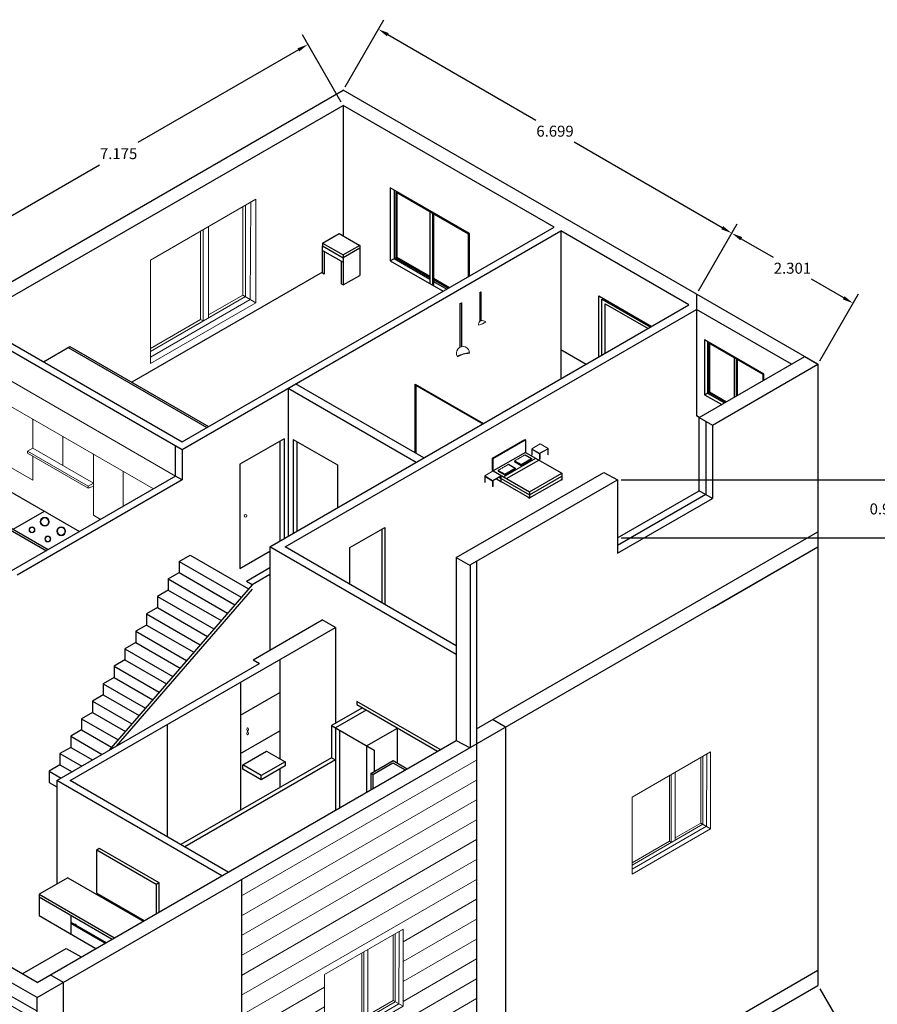
# Model space of a CAD drawing. Units: metres. Extents: x 14054 to 28215, y 4175 to 8383.
# Tile 3 of 6: x 14063.29 to 14077.36, y 4183.08 to 4199.25. Entities that reach past the tile are written whole.
import ezdxf

# ---------------------------------------------------------------- set-up
doc = ezdxf.new("R2010")
doc.units = ezdxf.units.M
for name, color, linetype, lineweight in [('A-ANNO-DIMS', 2, 'Continuous', 18), ('A-ANNO-NPLT', 9, 'Continuous', 13), ('A-ELEV-ISOM', 7, 'Continuous', 25), ('A-FURN', 8, 'Continuous', 13), ('A-GLAZ', 4, 'Continuous', 18), ('A-WALL-PATT', 8, 'Continuous', 13)]:
    doc.layers.add(name, color=color, linetype=linetype, lineweight=lineweight)
doc.styles.get("Standard").update_dxf_attribs({"font": 'arial.ttf'})
doc.dimstyles.get("Standard").update_dxf_attribs({"dimtxt": 0.18, "dimasz": 0.18, "dimexe": 0.18, "dimexo": 0.0625, "dimgap": 0.09, "dimtad": 0, "dimtih": 1, "dimtoh": 1, "dimdec": 4, "dimzin": 0, "dimdsep": 46, "dimtxsty": 'Standard', "dimcen": 0.09, "dimadec": 0, "dimazin": 0, "dimtfac": 1, "dimtdec": 4, "dimtofl": 0, "dimtmove": 0, "dimatfit": 3, "dimfxl": 1, "dimtolj": 1, "dimtzin": 0, "dimarcsym": 0})

# ---------------------------------------------------------------- blocks, each defined once
blk = doc.blocks.new('WINDOWS')
for p, q in [((14062.382, 4194.254), (14062.382, 4193.754)), ((14062.382, 4193.754), (14062.017, 4193.543)), ((14062.382, 4193.754), (14065.846, 4191.754)), ((14062.017, 4193.543), (14065.481, 4191.543)), ((14062.017, 4193.543), (14062.017, 4192.543)), ((14062.512, 4193.258), (14062.512, 4192.258)), ((14063.007, 4192.972), (14063.007, 4191.972)), ((14063.502, 4192.686), (14063.502, 4192.214)), ((14062.017, 4192.543), (14063.502, 4191.686)), ((14062.187, 4192.446), (14062.187, 4192.046)), ((14063.997, 4192.4), (14063.997, 4191.928)), ((14063.502, 4192.214), (14063.414, 4192.164)), ((14063.502, 4192.214), (14064.498, 4191.639)), ((14063.414, 4192.164), (14064.411, 4191.589)), ((14063.414, 4192.164), (14063.414, 4192.132)), ((14063.414, 4192.132), (14064.411, 4191.557)), ((14063.502, 4192.082), (14063.502, 4191.686)), ((14064.498, 4192.111), (14064.498, 4191.111)), ((14064.987, 4191.829), (14064.987, 4191.258)), ((14064.498, 4191.639), (14064.411, 4191.589)), ((14064.411, 4191.589), (14064.411, 4191.557)), ((14064.411, 4191.557), (14064.498, 4191.589)), ((14064.498, 4191.111), (14064.615, 4191.043))]:
    blk.add_line(p, q)
for p in [(14062.512, 4193.258), (14063.007, 4192.972), (14063.502, 4192.686), (14064.492, 4192.115), (14064.987, 4191.829)]:
    blk.add_point(p)
blk = doc.blocks.new('WINDOW 1')
for p, q in [((14073.717, 4186.789), (14075.449, 4187.789)), ((14075.276, 4187.689), (14075.276, 4186.189)), ((14075.365, 4187.74), (14075.356, 4186.143)), ((14075.449, 4187.789), (14075.449, 4186.089)), ((14075.233, 4187.664), (14075.233, 4186.214)), ((14074.54, 4187.264), (14074.54, 4185.814)), ((14074.583, 4187.289), (14074.583, 4185.789)), ((14074.67, 4187.34), (14074.67, 4185.84)), ((14073.717, 4185.089), (14073.717, 4186.789)), ((14075.276, 4186.189), (14073.717, 4185.289)), ((14075.356, 4186.143), (14073.717, 4185.197)), ((14075.449, 4186.089), (14073.717, 4185.089)), ((14075.233, 4186.214), (14074.67, 4185.889)), ((14075.233, 4186.214), (14075.449, 4186.089)), ((14074.54, 4185.814), (14073.717, 4185.339)), ((14074.583, 4185.789), (14074.54, 4185.814))]:
    blk.add_line(p, q)
blk = doc.blocks.new('TABLE')
for p, q in [((14070.836, 4191.718), (14070.938, 4191.777)), ((14070.938, 4191.777), (14071.033, 4191.722)), ((14070.836, 4191.718), (14070.93, 4191.663)), ((14070.836, 4191.718), (14070.836, 4191.711)), ((14070.836, 4191.711), (14070.93, 4191.656)), ((14070.836, 4191.711), (14070.836, 4191.643)), ((14070.841, 4191.64), (14070.836, 4191.643)), ((14070.841, 4191.708), (14070.841, 4191.64)), ((14071.033, 4191.722), (14070.93, 4191.663)), ((14071.033, 4191.715), (14070.93, 4191.656)), ((14070.93, 4191.656), (14070.93, 4191.663)), ((14070.93, 4191.589), (14070.93, 4191.656)), ((14070.937, 4191.66), (14070.937, 4191.592)), ((14071.027, 4191.644), (14071.027, 4191.712)), ((14071.033, 4191.648), (14071.027, 4191.644)), ((14071.033, 4191.722), (14071.033, 4191.715)), ((14071.033, 4191.715), (14071.033, 4191.648)), ((14070.937, 4191.592), (14070.93, 4191.589))]:
    blk.add_line(p, q)
blk = doc.blocks.new('*D11')
at = {"layer": 'A-ANNO-DIMS', "color": 0, "lineweight": -2, "transparency": 16777216}
for p, q in [((14076.421, 4183.337), (14077.057, 4182.235)), ((14076.812, 4182.301), (14070.874, 4178.873)), ((14064.306, 4175.081), (14070.244, 4178.509)), ((14063.604, 4175.937), (14064.24, 4174.835))]:
    blk.add_line(p, q, dxfattribs=at)
at = {"layer": 'A-ANNO-DIMS', "color": 0, "transparency": 16777216}
for points in [[(14076.797, 4182.327), (14076.827, 4182.275), (14076.967, 4182.391)], [(14064.291, 4175.107), (14064.321, 4175.055), (14064.15, 4174.991)]]:
    blk.add_solid(points, dxfattribs=at)
at = {"layer": 'Defpoints', "color": 0, "transparency": 16777216}
for p in [(14076.39, 4183.391), (14063.573, 4175.991), (14064.15, 4174.991)]:
    blk.add_point(p, dxfattribs=at)
at = {"layer": 'A-ANNO-DIMS', "color": 0, "transparency": 16777216, "insert": (14070.559, 4178.691), "char_height": 0.18, "attachment_point": 5}
blk.add_mtext('\\A1;14.8', dxfattribs=at)
blk = doc.blocks.new('*D72')
at = {"layer": 'A-ANNO-DIMS', "color": 0, "lineweight": -2, "transparency": 16777216}
for p, q in [((14068.564, 4197.895), (14067.928, 4198.997)), ((14067.862, 4198.752), (14065.226, 4197.23)), ((14061.96, 4195.344), (14064.596, 4196.866)), ((14062.351, 4194.308), (14061.714, 4195.41))]:
    blk.add_line(p, q, dxfattribs=at)
at = {"layer": 'A-ANNO-DIMS', "color": 0, "transparency": 16777216}
for points in [[(14067.847, 4198.777), (14067.877, 4198.726), (14068.018, 4198.842)], [(14061.945, 4195.37), (14061.975, 4195.318), (14061.804, 4195.254)]]:
    blk.add_solid(points, dxfattribs=at)
at = {"layer": 'Defpoints', "color": 0, "transparency": 16777216}
for p in [(14068.018, 4198.842), (14068.596, 4197.841), (14062.382, 4194.254)]:
    blk.add_point(p, dxfattribs=at)
at = {"layer": 'A-ANNO-DIMS', "color": 0, "transparency": 16777216, "insert": (14064.911, 4197.048), "char_height": 0.18, "attachment_point": 5}
blk.add_mtext('\\A1;7.175', dxfattribs=at)
blk = doc.blocks.new('*D73')
at = {"layer": 'A-ANNO-DIMS', "color": 0, "lineweight": -2, "transparency": 16777216}
for p, q in [((14068.627, 4198.145), (14069.263, 4199.247)), ((14069.329, 4199.002), (14071.759, 4197.599)), ((14074.819, 4195.832), (14072.389, 4197.235)), ((14074.429, 4194.796), (14075.065, 4195.898))]:
    blk.add_line(p, q, dxfattribs=at)
at = {"layer": 'A-ANNO-DIMS', "color": 0, "transparency": 16777216}
for points in [[(14069.344, 4199.027), (14069.314, 4198.976), (14069.173, 4199.092)], [(14074.834, 4195.858), (14074.804, 4195.806), (14074.975, 4195.742)]]:
    blk.add_solid(points, dxfattribs=at)
at = {"layer": 'Defpoints', "color": 0, "transparency": 16777216}
for p in [(14068.596, 4198.091), (14074.975, 4195.742), (14074.397, 4194.742)]:
    blk.add_point(p, dxfattribs=at)
at = {"layer": 'A-ANNO-DIMS', "color": 0, "transparency": 16777216, "insert": (14072.074, 4197.417), "char_height": 0.18, "attachment_point": 5}
blk.add_mtext('\\A1;6.699', dxfattribs=at)
blk = doc.blocks.new('*D74')
at = {"layer": 'A-ANNO-DIMS', "color": 0, "lineweight": -2, "transparency": 16777216}
for p, q in [((14074.429, 4194.796), (14075.065, 4195.898)), ((14075.131, 4195.652), (14075.656, 4195.349)), ((14076.812, 4194.682), (14076.286, 4194.985)), ((14076.421, 4193.645), (14077.057, 4194.747))]:
    blk.add_line(p, q, dxfattribs=at)
at = {"layer": 'A-ANNO-DIMS', "color": 0, "transparency": 16777216}
for points in [[(14075.146, 4195.678), (14075.116, 4195.626), (14074.975, 4195.742)], [(14076.827, 4194.707), (14076.797, 4194.656), (14076.967, 4194.592)]]:
    blk.add_solid(points, dxfattribs=at)
at = {"layer": 'Defpoints', "color": 0, "transparency": 16777216}
for p in [(14074.397, 4194.742), (14076.967, 4194.592), (14076.39, 4193.591)]:
    blk.add_point(p, dxfattribs=at)
at = {"layer": 'A-ANNO-DIMS', "color": 0, "transparency": 16777216, "insert": (14075.971, 4195.167), "char_height": 0.18, "attachment_point": 5}
blk.add_mtext('\\A1;2.301', dxfattribs=at)
blk = doc.blocks.new('*D75')
at = {"layer": 'A-ANNO-DIMS', "color": 0, "lineweight": -2, "transparency": 16777216}
for p, q in [((14073.161, 4191.691), (14077.725, 4191.691)), ((14077.545, 4191.511), (14077.545, 4191.397)), ((14077.545, 4190.918), (14077.545, 4191.033)), ((14073.161, 4190.738), (14077.725, 4190.738))]:
    blk.add_line(p, q, dxfattribs=at)
at = {"layer": 'A-ANNO-DIMS', "color": 0, "transparency": 16777216}
for points in [[(14077.515, 4191.511), (14077.575, 4191.511), (14077.545, 4191.691)], [(14077.515, 4190.918), (14077.575, 4190.918), (14077.545, 4190.738)]]:
    blk.add_solid(points, dxfattribs=at)
at = {"layer": 'Defpoints', "color": 0, "transparency": 16777216}
for p in [(14073.099, 4191.691), (14073.099, 4190.738), (14077.545, 4190.738)]:
    blk.add_point(p, dxfattribs=at)
at = {"layer": 'A-ANNO-DIMS', "color": 0, "transparency": 16777216, "insert": (14077.545, 4191.215), "char_height": 0.18, "attachment_point": 5}
blk.add_mtext('\\A1;0.953', dxfattribs=at)

msp = doc.modelspace()

# ---------------------------------------------------------------- hatches: boundary and pattern name
at = {"layer": 'A-WALL-PATT'}
h = msp.add_hatch(dxfattribs=at)
h.set_pattern_fill('ANSI38', color=256, scale=0.092, angle=105)
h.paths.add_polyline_path([(14055.7785, 4187.4672), (14055.7785, 4180.7413), (14058.8262, 4178.9816), (14058.8262, 4185.7075)])
h.paths.add_polyline_path([(14058.0676, 4184.5273), (14058.0676, 4183.2595), (14056.6953, 4184.0519), (14056.6953, 4185.3196)], flags=16)
h.paths.add_polyline_path([(14056.7604, 4184.0895), (14056.7893, 4184.1061), (14056.7893, 4185.2436), (14058.0488, 4184.5164), (14058.0488, 4183.401), (14057.4455, 4183.7494), (14057.4455, 4183.6399), (14057.4272, 4183.6293), (14057.4272, 4184.8753), (14057.3815, 4184.9017), (14057.3815, 4183.7309)], flags=0)
h.paths.add_polyline_path([(14063.5727, 4180.0812), (14062.8942, 4180.4729), (14061.5218, 4181.2653), (14060.8587, 4181.6535), (14060.8401, 4177.8243), (14063.5727, 4176.2413)])
h.paths.add_polyline_path([(14060.8494, 4184.7636), (14060.9576, 4184.8261), (14058.9345, 4185.9941), (14058.9345, 4178.9191), (14060.8494, 4177.8136)])
h.paths.add_polyline_path([(14060.7529, 4181.7978), (14060.7529, 4181.7242), (14060.7529, 4178.127), (14059.0613, 4179.1036), (14059.0613, 4182.7744)], flags=16)
h.paths.add_polyline_path([(14059.2399, 4179.1538), (14059.2399, 4182.5977), (14060.0427, 4182.1342), (14060.0427, 4178.6903)], flags=0)
h.paths.add_polyline_path([(14060.215, 4182.0347), (14060.7096, 4181.7492), (14060.7096, 4178.3053), (14060.215, 4178.5908)], flags=0)
edge = h.paths.add_edge_path(flags=0)
edge.add_ellipse((14059.9307, 4180.1763), major_axis=(-0.0333, 0.0192), ratio=0.8810932, start_angle=0, end_angle=360)
h = msp.add_hatch(dxfattribs=at)
h.set_pattern_fill('ANSI31', color=256, scale=0.089, angle=165)
h.paths.add_polyline_path([(14070.7875, 4187.3567), (14066.9286, 4185.1288), (14066.9286, 4178.1788), (14070.7875, 4180.4067)])
h.paths.add_polyline_path([(14069.5808, 4184.3152), (14069.5808, 4183.05), (14068.2917, 4182.3057), (14068.2917, 4183.5709)], flags=16)
h.paths.add_polyline_path([(14069.4519, 4183.1244), (14069.0007, 4182.8639), (14069.0007, 4182.9011), (14069.4197, 4183.143)], flags=0)
h = msp.add_hatch(dxfattribs=at)
h.set_pattern_fill('ANSI31', color=256, scale=0.089, angle=105)
h.paths.add_polyline_path([(14063.5727, 4182.9672), (14060.8494, 4184.5395), (14060.8494, 4181.6535), (14061.5218, 4181.2653), (14061.5218, 4182.533), (14062.8942, 4181.7407), (14062.8942, 4180.4729), (14063.5727, 4180.0812)])

# ---------------------------------------------------------------- linework, layer by layer
at = {"layer": 'A-ANNO-NPLT'}
msp.add_point((14063.9968, 4192.4004), dxfattribs=at)
at = {"layer": 'A-ELEV-ISOM'}
for p, q in [((14055.995, 4190.8163), (14068.5957, 4198.0913)), ((14076.3899, 4193.5913), (14068.5957, 4198.0913)), ((14062.4902, 4194.3163), (14068.5957, 4197.8413)), ((14072.0598, 4195.8413), (14068.5957, 4197.8413)), ((14068.5957, 4197.8413), (14068.5957, 4195.6998)), ((14070.6694, 4195.7385), (14069.3703, 4196.4885)), ((14069.3703, 4196.4885), (14069.3703, 4195.2885)), ((14069.4319, 4196.4529), (14069.4319, 4195.3241)), ((14069.4593, 4196.4166), (14069.4593, 4195.3399)), ((14070.6515, 4195.7282), (14069.4593, 4196.4166)), ((14069.4774, 4196.4061), (14069.4774, 4195.3503)), ((14070.0198, 4196.0929), (14070.0198, 4194.9135)), ((14070.0631, 4196.0679), (14070.0631, 4194.8885)), ((14070.0805, 4196.0579), (14070.0805, 4194.8985)), ((14065.9543, 4192.3163), (14072.0598, 4195.8413)), ((14065.9543, 4192.1913), (14072.168, 4195.7788)), ((14074.2724, 4194.5638), (14072.168, 4195.7788)), ((14072.168, 4195.7788), (14072.168, 4193.3489)), ((14068.2589, 4195.5789), (14068.5321, 4195.7366)), ((14068.5321, 4195.7366), (14068.8682, 4195.5425)), ((14070.6515, 4195.0282), (14070.6515, 4195.7282)), ((14070.6694, 4195.0385), (14070.6694, 4195.7385)), ((14068.2589, 4195.5789), (14068.595, 4195.3848)), ((14068.2589, 4195.5789), (14068.2589, 4195.5335)), ((14068.2589, 4195.5335), (14068.595, 4195.3395)), ((14068.2589, 4195.0861), (14068.2589, 4195.5335)), ((14068.2589, 4195.46), (14068.595, 4195.266)), ((14068.2836, 4195.4458), (14068.2836, 4195.0719)), ((14068.8682, 4195.5425), (14068.595, 4195.3848)), ((14068.8682, 4195.4972), (14068.595, 4195.3395)), ((14068.8682, 4195.5425), (14068.8682, 4195.4972)), ((14068.8682, 4195.4972), (14068.8682, 4195.0498)), ((14068.5703, 4194.9063), (14068.5703, 4195.2802)), ((14068.595, 4195.3848), (14068.595, 4195.3395)), ((14068.595, 4195.3395), (14068.595, 4194.8921)), ((14069.3703, 4195.2885), (14069.4774, 4195.3503)), ((14069.3703, 4195.2885), (14070.2363, 4194.7885)), ((14069.4319, 4195.3241), (14070.0198, 4194.9847)), ((14069.4593, 4195.3399), (14070.0198, 4195.0163)), ((14069.4774, 4195.3503), (14070.0198, 4195.0372)), ((14068.2589, 4195.1038), (14065.1255, 4193.2947)), ((14068.2836, 4195.0719), (14068.2589, 4195.0861)), ((14068.595, 4194.8921), (14068.8682, 4195.0498)), ((14070.0805, 4195.0022), (14070.3434, 4194.8503)), ((14070.0805, 4194.9813), (14070.3253, 4194.8399)), ((14070.0805, 4194.9497), (14070.298, 4194.8241)), ((14068.595, 4194.8921), (14068.5703, 4194.9063)), ((14070.0631, 4194.8885), (14070.0805, 4194.8985)), ((14070.8402, 4194.7666), (14070.861, 4194.7786)), ((14070.8402, 4194.7666), (14070.8402, 4194.2979)), ((14070.861, 4194.3098), (14070.861, 4194.7786)), ((14072.7947, 4193.7107), (14072.7947, 4194.7144)), ((14072.7947, 4194.7144), (14073.6639, 4194.2125)), ((14072.8405, 4193.7371), (14072.8405, 4194.6593)), ((14072.8405, 4194.6593), (14073.6391, 4194.1982)), ((14074.3974, 4194.7416), (14074.3974, 4192.7428)), ((14067.3937, 4190.5924), (14074.2724, 4194.5638)), ((14067.6437, 4190.5924), (14074.3974, 4194.4916)), ((14070.5109, 4194.583), (14070.5109, 4193.8679)), ((14070.5389, 4194.5992), (14070.5389, 4193.8786)), ((14072.8959, 4193.7691), (14072.8959, 4194.5826)), ((14072.8959, 4194.5826), (14073.6004, 4194.1759)), ((14075.9569, 4193.5913), (14074.3974, 4194.4916)), ((14062.4902, 4194.3163), (14065.9543, 4192.3163)), ((14070.8402, 4194.2979), (14070.861, 4194.3098)), ((14062.3819, 4194.2538), (14065.9543, 4192.1913)), ((14075.5034, 4193.4278), (14074.5303, 4193.9896)), ((14074.5303, 4193.9896), (14074.5303, 4193.0907)), ((14063.6782, 4193.6303), (14064.1113, 4193.8803)), ((14064.0839, 4193.8645), (14066.3599, 4192.5505)), ((14064.1113, 4193.8803), (14066.3873, 4192.5663)), ((14072.168, 4193.8328), (14072.5871, 4193.5909)), ((14074.5764, 4193.963), (14074.5764, 4193.1174)), ((14074.5969, 4193.9357), (14074.5969, 4193.1292)), ((14075.4901, 4193.4201), (14074.5969, 4193.9357)), ((14074.6105, 4193.9279), (14074.6105, 4193.137)), ((14074.4413, 4192.7163), (14076.1734, 4193.7163)), ((14075.0168, 4193.6933), (14075.0168, 4193.0485)), ((14075.0493, 4193.6746), (14075.0493, 4193.0673)), ((14075.0622, 4193.6671), (14075.0622, 4193.0747)), ((14076.1734, 4193.7163), (14076.3899, 4193.5913)), ((14074.6578, 4192.5913), (14076.3899, 4193.5913)), ((14076.3899, 4193.5913), (14076.3899, 4190.5913)), ((14075.4901, 4193.3217), (14075.4901, 4193.4201)), ((14075.5034, 4193.3294), (14075.5034, 4193.4278)), ((14069.7963, 4191.9795), (14067.6919, 4193.1945)), ((14067.6919, 4193.1945), (14067.6919, 4190.7646)), ((14069.9213, 4192.0517), (14067.8169, 4193.2666)), ((14069.7798, 4192.1334), (14069.7798, 4193.2657)), ((14069.7798, 4193.2657), (14070.9018, 4192.6179)), ((14069.7933, 4193.2434), (14070.8893, 4192.6106)), ((14069.7933, 4192.1256), (14069.7933, 4193.2434)), ((14074.5303, 4193.0907), (14074.6105, 4193.137)), ((14074.5303, 4193.0907), (14074.8101, 4192.9292)), ((14074.5764, 4193.1174), (14074.8562, 4192.9558)), ((14074.5969, 4193.1292), (14074.8767, 4192.9676)), ((14074.6105, 4193.137), (14074.8903, 4192.9755)), ((14074.4413, 4192.7163), (14074.3974, 4192.7428)), ((14074.4413, 4191.5132), (14074.4413, 4192.7163)), ((14074.4413, 4192.7163), (14074.6578, 4192.5913)), ((14074.5496, 4192.6538), (14074.5496, 4191.4507)), ((14074.6578, 4192.5913), (14074.6578, 4191.3882)), ((14067.6262, 4192.3666), (14066.903, 4191.949)), ((14067.6262, 4192.3666), (14067.6262, 4190.7267)), ((14065.846, 4191.7538), (14065.846, 4192.2538)), ((14067.5562, 4192.3261), (14067.5562, 4190.6862)), ((14067.7759, 4192.356), (14068.5011, 4191.9373)), ((14067.7759, 4192.356), (14067.7759, 4190.8131)), ((14067.838, 4192.3202), (14067.838, 4190.8489)), ((14071.0498, 4192.0485), (14071.5783, 4192.3536)), ((14071.0605, 4192.0423), (14071.589, 4192.3474)), ((14071.5783, 4192.3536), (14071.589, 4192.3474)), ((14071.589, 4192.3474), (14071.589, 4192.144)), ((14062.1865, 4192.0456), (14064.269, 4190.8433)), ((14065.9543, 4192.1913), (14065.9543, 4191.6913)), ((14071.0498, 4191.8451), (14071.0498, 4192.0485)), ((14071.0605, 4192.0423), (14071.0498, 4192.0485)), ((14071.589, 4192.144), (14071.0605, 4191.8389)), ((14071.0605, 4191.8389), (14071.0605, 4192.0423)), ((14071.2285, 4191.7419), (14071.757, 4192.047)), ((14071.5184, 4191.9427), (14071.6903, 4192.0419)), ((14071.583, 4192.1038), (14071.6903, 4192.0419)), ((14071.589, 4192.144), (14072.1834, 4191.8008)), ((14071.6903, 4192.0419), (14071.6903, 4192.0295)), ((14066.903, 4191.949), (14066.903, 4190.2376)), ((14068.5011, 4191.9373), (14068.5011, 4191.2318)), ((14071.248, 4191.7866), (14071.4199, 4191.8858)), ((14071.2788, 4191.7129), (14071.8072, 4192.018)), ((14071.3126, 4191.9477), (14071.4199, 4191.8858)), ((14071.4111, 4192.0046), (14071.5184, 4191.9427)), ((14071.4111, 4192.0046), (14071.4111, 4191.9922)), ((14071.4111, 4191.9922), (14071.5184, 4191.9302)), ((14071.4199, 4191.8858), (14071.4199, 4191.8734)), ((14071.5184, 4191.9302), (14071.6903, 4192.0295)), ((14071.5184, 4191.9302), (14071.5184, 4191.9427)), ((14065.846, 4191.7538), (14063.1397, 4190.1913)), ((14065.9543, 4191.6913), (14065.846, 4191.7538)), ((14070.4541, 4190.4158), (14072.8739, 4191.8121)), ((14071.0498, 4191.8451), (14071.0605, 4191.8389)), ((14071.0605, 4191.8389), (14071.6549, 4191.4957)), ((14071.1408, 4191.8485), (14071.248, 4191.7866)), ((14071.1408, 4191.8485), (14071.1408, 4191.8361)), ((14071.1408, 4191.8361), (14071.248, 4191.7741)), ((14071.1551, 4191.7342), (14071.1817, 4191.7189)), ((14071.248, 4191.7741), (14071.4199, 4191.8734)), ((14071.248, 4191.7741), (14071.248, 4191.7866)), ((14071.6549, 4191.4957), (14072.1834, 4191.8008)), ((14071.6549, 4191.4457), (14072.1834, 4191.7508)), ((14072.1834, 4191.8008), (14072.1834, 4191.7008)), ((14072.8739, 4191.8121), (14073.099, 4191.6913)), ((14065.9543, 4191.6913), (14063.248, 4190.1288)), ((14070.6792, 4190.295), (14073.099, 4191.6913)), ((14071.1118, 4191.7092), (14071.1817, 4191.6689)), ((14071.1901, 4191.7141), (14071.6549, 4191.4457)), ((14071.1901, 4191.6641), (14071.6549, 4191.3957)), ((14071.6549, 4191.3957), (14072.1834, 4191.7008)), ((14072.1834, 4191.6894), (14072.1735, 4191.6951)), ((14072.1834, 4191.7008), (14072.1834, 4191.6894)), ((14073.099, 4191.6913), (14073.099, 4190.4882)), ((14062.1761, 4191.4597), (14063.7564, 4190.5473)), ((14062.1761, 4191.4245), (14063.7259, 4190.5297)), ((14071.6369, 4191.3978), (14071.6369, 4191.4061)), ((14071.6549, 4191.3874), (14071.6369, 4191.3978)), ((14071.6549, 4191.4957), (14071.6549, 4191.3957)), ((14071.6549, 4191.3957), (14071.6549, 4191.3874)), ((14073.099, 4190.7382), (14074.4413, 4191.5132)), ((14074.5496, 4191.4507), (14073.099, 4190.6132)), ((14074.6578, 4191.3882), (14074.4413, 4191.5132)), ((14073.099, 4190.4882), (14074.6578, 4191.3882)), ((14063.1795, 4190.8803), (14063.6922, 4191.1763)), ((14068.7054, 4190.5795), (14069.2802, 4190.9114)), ((14069.2802, 4190.9114), (14069.2802, 4189.6476)), ((14069.2309, 4190.8829), (14069.2309, 4189.6761)), ((14070.7875, 4187.6067), (14076.3899, 4190.8413)), ((14063.5727, 4183.1913), (14076.3899, 4190.5913)), ((14070.4541, 4188.8255), (14067.3937, 4190.5924)), ((14067.3937, 4190.5924), (14067.3937, 4188.8987)), ((14070.4541, 4188.9698), (14067.6437, 4190.5924)), ((14071.2638, 4190.6325), (14071.2638, 4190.6323)), ((14074.6578, 4189.5913), (14076.3899, 4190.5913)), ((14076.3899, 4190.5913), (14076.3899, 4183.3913)), ((14065.9049, 4190.3536), (14066.0829, 4190.4564)), ((14066.0829, 4190.4564), (14067.0425, 4189.9024)), ((14066.903, 4190.2376), (14067.3937, 4190.5209)), ((14068.7054, 4189.9795), (14068.7054, 4190.5795)), ((14065.9049, 4190.3536), (14066.924, 4189.7652)), ((14065.9049, 4190.3536), (14065.9049, 4190.1695)), ((14070.4541, 4190.4158), (14070.4541, 4187.415)), ((14070.4541, 4190.4158), (14070.6792, 4190.2859)), ((14070.6792, 4190.295), (14070.6792, 4187.2942)), ((14070.7875, 4190.3575), (14070.7875, 4180.4067)), ((14065.7269, 4190.0667), (14065.9049, 4190.1695)), ((14065.9049, 4190.1695), (14066.8179, 4189.6423)), ((14065.9049, 4190.1695), (14066.7713, 4189.6692)), ((14067.3937, 4190.2457), (14067.0101, 4190.0242)), ((14067.3937, 4190.1397), (14067.1019, 4189.9712)), ((14067.1019, 4189.9712), (14064.7492, 4187.2466)), ((14065.7269, 4190.0667), (14066.6995, 4189.5052)), ((14065.7269, 4190.0667), (14065.7269, 4189.8825)), ((14067.1019, 4189.9712), (14067.0101, 4190.0242)), ((14067.1019, 4189.8997), (14064.8724, 4187.3177)), ((14065.7269, 4189.8825), (14065.5489, 4189.7798)), ((14065.5489, 4189.7798), (14066.4749, 4189.2451)), ((14065.5489, 4189.7798), (14065.5489, 4189.5956)), ((14065.7269, 4189.8825), (14066.5933, 4189.3823)), ((14065.7269, 4189.8825), (14066.5933, 4189.3823)), ((14065.5489, 4189.5956), (14065.3709, 4189.4928)), ((14065.3709, 4189.4928), (14066.2504, 4188.9851)), ((14065.3709, 4189.4928), (14065.3709, 4189.3086)), ((14065.5489, 4189.5956), (14066.3688, 4189.1222)), ((14065.3709, 4189.3086), (14065.1929, 4189.2059)), ((14065.3709, 4189.3086), (14066.1442, 4188.8622)), ((14067.1171, 4188.739), (14068.2516, 4189.394)), ((14068.4686, 4189.2687), (14068.2516, 4189.394)), ((14064.1133, 4186.7541), (14068.4686, 4189.2687)), ((14065.1929, 4189.2059), (14066.0258, 4188.725)), ((14065.1929, 4189.2059), (14065.1929, 4189.0217)), ((14068.4686, 4189.2687), (14068.4686, 4187.6936)), ((14065.1929, 4189.0217), (14065.0149, 4188.9189)), ((14065.1929, 4189.0217), (14065.9197, 4188.6021)), ((14065.0149, 4188.9189), (14065.8012, 4188.4649)), ((14065.0149, 4188.9189), (14065.0149, 4188.7348)), ((14063.8965, 4186.7543), (14067.2256, 4188.6763)), ((14065.0149, 4188.7348), (14064.8369, 4188.632)), ((14065.0149, 4188.7348), (14065.6951, 4188.342)), ((14067.1171, 4188.739), (14067.2256, 4188.6763)), ((14067.5552, 4188.7413), (14067.5552, 4187.1123)), ((14064.8369, 4188.632), (14065.5767, 4188.2049)), ((14064.8369, 4188.632), (14064.8369, 4188.4478)), ((14064.8369, 4188.4478), (14064.6589, 4188.3451)), ((14064.6589, 4188.3451), (14065.3521, 4187.9448)), ((14064.6589, 4188.3451), (14064.6589, 4188.1609)), ((14064.8369, 4188.4478), (14065.4705, 4188.082)), ((14066.9135, 4188.3708), (14066.9135, 4186.2691)), ((14064.6589, 4188.1609), (14064.4809, 4188.0581)), ((14064.6589, 4188.1609), (14065.246, 4187.8219)), ((14066.9135, 4187.8312), (14067.5552, 4188.2017)), ((14064.4809, 4188.0581), (14065.1276, 4187.6848)), ((14064.4809, 4188.0581), (14064.4809, 4187.8739)), ((14070.1907, 4187.2629), (14068.8222, 4188.053)), ((14068.8222, 4188.053), (14068.8222, 4188.0015)), ((14068.8222, 4188.0015), (14070.146, 4187.2371)), ((14064.4809, 4187.8739), (14064.3029, 4187.7712)), ((14064.4809, 4187.8739), (14065.0214, 4187.5619)), ((14068.912, 4187.9496), (14068.4052, 4187.657)), ((14068.9754, 4187.913), (14068.4686, 4187.6204)), ((14064.3029, 4187.7712), (14064.903, 4187.4247)), ((14064.3029, 4187.7712), (14064.3029, 4187.587)), ((14065.7061, 4187.6737), (14065.7061, 4185.8346)), ((14071.2638, 4187.6317), (14071.0473, 4187.7567)), ((14064.3029, 4187.587), (14064.1249, 4187.4842)), ((14064.3029, 4187.587), (14064.7969, 4187.3018)), ((14066.9135, 4187.2024), (14067.5552, 4187.5728)), ((14068.4052, 4187.657), (14069.1041, 4187.2535)), ((14068.4052, 4187.657), (14068.4052, 4187.1304)), ((14068.4686, 4187.6204), (14068.4686, 4186.2687)), ((14068.5346, 4187.5823), (14068.5346, 4186.3068)), ((14068.9806, 4187.3248), (14069.4874, 4187.6174)), ((14069.4841, 4187.6193), (14069.4841, 4187.0451)), ((14071.2638, 4187.6317), (14071.2638, 4180.6817)), ((14063.572, 4183.4416), (14070.4541, 4187.415)), ((14064.1249, 4187.4842), (14064.6429, 4187.1852)), ((14064.1249, 4187.4842), (14064.1249, 4187.3001)), ((14070.4541, 4187.415), (14070.6792, 4187.2942)), ((14064.1249, 4187.3001), (14063.9469, 4187.1973)), ((14063.9469, 4187.1973), (14064.3054, 4186.9903)), ((14063.9469, 4187.1973), (14063.9469, 4187.0131)), ((14064.1249, 4187.3001), (14064.4834, 4187.0931)), ((14064.1249, 4187.3001), (14064.4834, 4187.0931)), ((14066.95, 4187.0109), (14067.3404, 4187.2363)), ((14067.3404, 4187.2363), (14067.6428, 4187.0617)), ((14068.9806, 4187.3248), (14068.9806, 4186.5643)), ((14069.1041, 4187.2535), (14069.1041, 4186.9023)), ((14068.4052, 4187.1304), (14065.9334, 4185.7033)), ((14068.4686, 4187.0938), (14065.9968, 4185.6667)), ((14067.6428, 4187.0617), (14067.2525, 4186.8363)), ((14067.6428, 4187.0617), (14067.6428, 4186.9949)), ((14068.4052, 4187.1304), (14068.4686, 4187.0938)), ((14069.0516, 4186.872), (14069.4178, 4187.0834)), ((14069.0821, 4186.8544), (14069.4133, 4187.0457)), ((14069.4133, 4187.0457), (14069.6139, 4186.9299)), ((14069.4178, 4187.0834), (14069.6488, 4186.95)), ((14063.9469, 4187.0131), (14063.7689, 4186.9103)), ((14063.7689, 4186.9103), (14063.9679, 4186.7955)), ((14063.7689, 4186.9103), (14063.7689, 4186.7262)), ((14063.9469, 4187.0131), (14064.1459, 4186.8982)), ((14067.2525, 4186.8363), (14066.95, 4187.0109)), ((14066.95, 4186.9441), (14066.95, 4187.0109)), ((14067.2525, 4186.7695), (14066.95, 4186.9441)), ((14067.6428, 4186.9949), (14067.2525, 4186.7695)), ((14067.5552, 4186.9443), (14067.5552, 4186.6396)), ((14069.0821, 4186.8544), (14069.0516, 4186.872)), ((14069.0516, 4186.872), (14069.0516, 4186.6053)), ((14063.572, 4183.4416), (14057.727, 4186.8163)), ((14063.7689, 4186.7262), (14063.8965, 4186.6525)), ((14063.7689, 4186.7262), (14063.8965, 4186.6525)), ((14066.6031, 4185.1916), (14063.8965, 4186.7543)), ((14063.8965, 4186.7543), (14063.8965, 4185.0573)), ((14066.7114, 4185.2541), (14064.1133, 4186.7541)), ((14067.2525, 4186.7695), (14067.2525, 4186.8363)), ((14069.0821, 4186.8544), (14069.0821, 4186.6229)), ((14064.5508, 4185.6196), (14064.5941, 4185.6446)), ((14064.5508, 4184.9089), (14064.5508, 4185.6196)), ((14064.5508, 4185.6196), (14065.5298, 4185.0544)), ((14064.5941, 4185.6446), (14065.5731, 4185.0794)), ((14064.0755, 4185.1606), (14063.6046, 4184.8888)), ((14064.0755, 4185.1606), (14065.3125, 4184.4465)), ((14066.9286, 4185.1288), (14066.9286, 4178.1788)), ((14065.5298, 4185.0544), (14065.5731, 4185.0794)), ((14065.5298, 4185.0544), (14065.5298, 4184.572)), ((14065.5731, 4185.0794), (14065.5731, 4184.597)), ((14063.5727, 4183.1913), (14060.8494, 4184.7636)), ((14063.6046, 4184.8888), (14064.8416, 4184.1746)), ((14063.6046, 4184.8888), (14063.6046, 4184.5399)), ((14063.6046, 4184.8468), (14064.8052, 4184.1536)), ((14064.5508, 4184.9089), (14065.3321, 4184.4578)), ((14063.5727, 4182.9672), (14060.8494, 4184.5395)), ((14063.6046, 4184.5399), (14064.5394, 4184.0002)), ((14064.1253, 4184.5461), (14064.1253, 4184.2393)), ((14064.1253, 4184.4296), (14064.7043, 4184.0954)), ((14064.1253, 4184.4154), (14064.6854, 4184.0921)), ((14064.1902, 4184.3922), (14064.1902, 4184.4056)), ((14064.1902, 4184.4056), (14064.2096, 4184.3945)), ((14064.2096, 4184.3945), (14064.2096, 4184.381)), ((14063.3269, 4183.5832), (14064.0498, 4184.0006)), ((14064.0498, 4184.0006), (14064.295, 4183.859)), ((14063.5727, 4176.2413), (14076.3899, 4183.6413)), ((14064.0057, 4183.4413), (14063.7885, 4183.5666)), ((14063.5727, 4175.9913), (14076.3899, 4183.3913)), ((14064.0057, 4176.2413), (14064.0057, 4183.4413)), ((14063.5727, 4175.9913), (14063.5727, 4183.1913))]:
    msp.add_line(p, q, dxfattribs=at)
at = {"layer": 'A-FURN'}
for centre, radius in [((14063.6993, 4191.0041), 0.0735), ((14066.9925, 4191.1028), 0.0218), ((14063.4894, 4190.8707), 0.0478), ((14063.4894, 4190.8707), 0.0407), ((14063.6993, 4191.0041), 0.0624), ((14063.9684, 4190.8487), 0.0735), ((14063.9684, 4190.8487), 0.0624), ((14063.748, 4190.7214), 0.0478), ((14063.748, 4190.7214), 0.0407)]:
    msp.add_circle(centre, radius, dxfattribs=at)
for centre, radius, start, end in [((14070.8385, 4194.082), 0.2289, 64.41331, 84.37459), ((14070.8896, 4194.2486), 0.0698, 135.11893, 192.82146), ((14070.7003, 4194.6356), 0.4204, 286.76902, 304.32774), ((14070.5633, 4193.7725), 0.1089, 359.46966, 214.04112), ((14070.6912, 4193.3441), 0.435, 92.53558, 120.5819), ((14070.6944, 4193.3371), 0.435, 92.92889, 120.5819)]:
    msp.add_arc(centre, radius, start, end, dxfattribs=at)
for centre, major_axis, ratio in [((14070.5249, 4194.5911), (-0.014, -0.0081), 0.1415216), ((14067.0289, 4187.5944), (0, 0.0266), 0.5527886), ((14067.0289, 4187.5307), (0, 0.0266), 0.5527886)]:
    msp.add_ellipse(centre, major_axis=major_axis, ratio=ratio, dxfattribs=at)
for points in [[(14071.4111, 4192.0046), (14071.4283, 4192.0145), (14071.4541, 4192.0294), (14071.4898, 4192.05), (14071.5136, 4192.0638), (14071.5373, 4192.0775), (14071.5539, 4192.087), (14071.5703, 4192.0965), (14071.578, 4192.101), (14071.583, 4192.1038)], [(14071.1408, 4191.8485), (14071.1579, 4191.8584), (14071.1837, 4191.8733), (14071.2194, 4191.8939), (14071.2432, 4191.9077), (14071.267, 4191.9214), (14071.2835, 4191.9309), (14071.2999, 4191.9404), (14071.3077, 4191.9449), (14071.3126, 4191.9477)]]:
    msp.add_open_spline(points, degree=3, knots=[0, 0, 0, 0, 0.05934304, 0.08933663, 0.12379449, 0.14166437, 0.17165796, 0.18123065, 0.19845639, 0.19845639, 0.19845639, 0.19845639], dxfattribs=at)

# ---------------------------------------------------------------- block references
at = {"layer": 'A-FURN', "xscale": 1.371911927489495, "yscale": 1.371911927489495, "zscale": 1.371911927489495}
for p in [(-5232.2556, -1558.4642), (-5233.0276, -1558.9099)]:
    msp.add_blockref('TABLE', p, dxfattribs=at)
at = {"layer": 'A-GLAZ'}
for name, p in [('WINDOW 1', (-8.2847, 8.5123)), ('WINDOWS', (0, 0))]:
    msp.add_blockref(name, p, dxfattribs=at)
at = {"layer": 'A-GLAZ', "xscale": 0.7442386112486127, "yscale": 0.7442386112486127, "zscale": 0.7442386112486127}
for p in [(3599.135, 1070.5149), (3594.088, 1067.601)]:
    msp.add_blockref('WINDOW 1', p, dxfattribs=at)

# ---------------------------------------------------------------- dimensions: what is measured, and where the dimension line sits
at = {"layer": 'A-ANNO-DIMS'}
for base, p1, p2, angle, override, picture, middle in [((14074.9749, 4195.7419), (14068.5957, 4198.0913), (14074.3974, 4194.7416), 330, {"dimdec": 3, "dimlfac": 1, "dimrnd": 0, "dimzin": 0, "dimdsep": 46, "dimlunit": 2}, '*D73', (14072.074, 4197.4167)), ((14068.0182, 4198.8415), (14062.3819, 4194.2538), (14068.5957, 4197.8413), 30, {"dimdec": 3, "dimlfac": 1, "dimrnd": 0, "dimzin": 0, "dimdsep": 46, "dimlunit": 2}, '*D72', (14064.9113, 4197.0478)), ((14076.9674, 4194.5915), (14074.3974, 4194.7416), (14076.3899, 4193.5913), 330, {"dimdec": 3, "dimlfac": 1, "dimrnd": 0, "dimzin": 0, "dimdsep": 46, "dimlunit": 2}, '*D74', (14075.9711, 4195.1667)), ((14077.5449, 4190.7382), (14073.099, 4191.6913), (14073.099, 4190.7382), 90, {"dimdec": 3, "dimlfac": 1, "dimrnd": 0, "dimzin": 0, "dimdsep": 46, "dimlunit": 2}, '*D75', (14077.5449, 4191.2147)), ((14064.1502, 4174.991), (14076.3899, 4183.3913), (14063.5727, 4175.9913), 210, {"dimdec": 1, "dimlfac": 1, "dimrnd": 0, "dimzin": 0, "dimdsep": 46, "dimlunit": 2}, '*D11', (14070.5588, 4178.691))]:
    dim = msp.add_linear_dim(base=base, p1=p1, p2=p2, angle=angle, dimstyle='Standard', override=override, dxfattribs=at)
    dim.commit()
    dim.dimension.update_dxf_attribs({"geometry": picture, "text_midpoint": middle})

doc.saveas('drawing.dxf')
